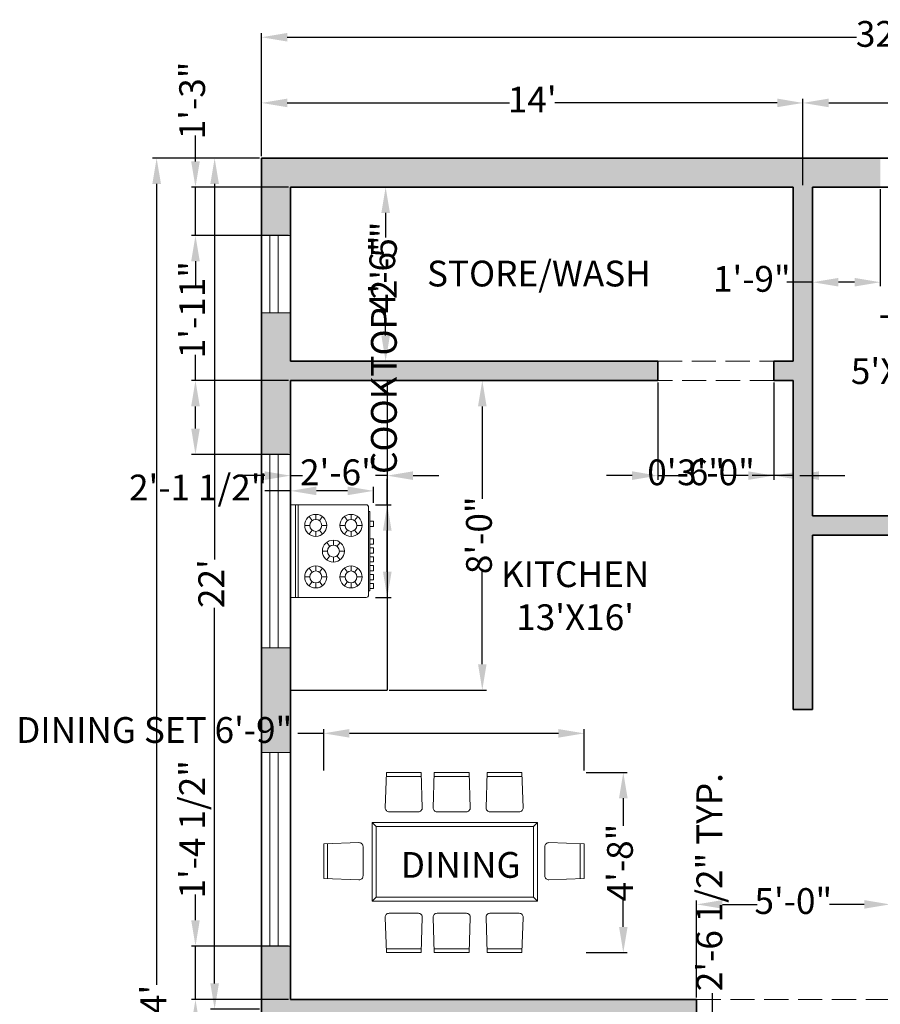
# Model space of a CAD drawing. Units: inches. Extents: x 2073 to 2646, y 2372 to 3017.
# Tile 4 of 8: x 2073 to 2340, y 2686 to 2992. Entities that reach past the tile are written whole.
import ezdxf

# ---------------------------------------------------------------- set-up
doc = ezdxf.new("R2010")
doc.units = ezdxf.units.IN
doc.linetypes.add('DASH', pattern=[0.35, 0.25, -0.1])
for name, color, linetype, lineweight in [('A-ANNO-DIMS', 2, 'Continuous', 18), ('A-AREA-IDEN', 7, 'Continuous', 25), ('A-EQPM', 8, 'Continuous', 18), ('A-FLOR-CASE', 8, 'Continuous', 25), ('A-FURN', 8, 'Continuous', 18), ('A-GLAZ', 4, 'Continuous', 18), ('A-WALL', 7, 'Continuous', 35), ('A-WALL-OVHD', 7, 'DASH', 18), ('A-WALL-PATT', 30, 'Continuous', 13)]:
    doc.layers.add(name, color=color, linetype=linetype, lineweight=lineweight)
doc.styles.get("Standard").update_dxf_attribs({"font": 'arial.ttf'})
doc.dimstyles.new('ISO-25', dxfattribs={"dimtxt": 8, "dimasz": 8, "dimexe": 1.25, "dimexo": 0.625, "dimtad": 0, "dimdec": 1, "dimlunit": 4, "dimtxsty": 'Standard', "dimcen": 2.5, "dimadec": 0, "dimazin": 0, "dimtfac": 1, "dimtdec": 1, "dimtmove": 0, "dimatfit": 3, "dimfxl": 1, "dimarcsym": 0})

# ---------------------------------------------------------------- blocks, each defined once
blk = doc.blocks.new('*D3')
at = {"layer": 'A-ANNO-DIMS', "color": 0, "lineweight": -2, "transparency": 16777216}
for p, q in [((2147.67, 2948.66), (2132.48, 2948.66)), ((2133.73, 2940.66), (2133.73, 2824.15)), ((2133.73, 2692.66), (2133.73, 2809.18)), ((2147.67, 2684.66), (2132.48, 2684.66))]:
    blk.add_line(p, q, dxfattribs=at)
at = {"layer": 'A-ANNO-DIMS', "color": 0, "transparency": 16777216}
for points in [[(2132.4, 2940.66), (2135.06, 2940.66), (2133.73, 2948.66)], [(2132.4, 2692.66), (2135.06, 2692.66), (2133.73, 2684.66)]]:
    blk.add_solid(points, dxfattribs=at)
at = {"layer": 'Defpoints', "color": 0, "transparency": 16777216}
for p in [(2133.73, 2948.66), (2148.29, 2948.66), (2148.29, 2684.66)]:
    blk.add_point(p, dxfattribs=at)
at = {"layer": 'A-ANNO-DIMS', "color": 0, "transparency": 16777216, "insert": (2133.73, 2816.66), "char_height": 8, "attachment_point": 5, "rotation": 90}
blk.add_mtext("22'", dxfattribs=at)
blk = doc.blocks.new('*D4')
at = {"layer": 'A-ANNO-DIMS', "color": 0, "lineweight": -2, "transparency": 16777216}
for p, q in [((2148.29, 2949.29), (2148.29, 2967.03)), ((2156.29, 2965.78), (2225.25, 2965.78)), ((2308.29, 2965.78), (2239.33, 2965.78)), ((2316.29, 2949.29), (2316.29, 2967.03))]:
    blk.add_line(p, q, dxfattribs=at)
at = {"layer": 'A-ANNO-DIMS', "color": 0, "transparency": 16777216}
for points in [[(2156.29, 2967.12), (2156.29, 2964.45), (2148.29, 2965.78)], [(2308.29, 2967.12), (2308.29, 2964.45), (2316.29, 2965.78)]]:
    blk.add_solid(points, dxfattribs=at)
at = {"layer": 'Defpoints', "color": 0, "transparency": 16777216}
for p in [(2316.29, 2965.78), (2148.29, 2948.66), (2316.29, 2948.66)]:
    blk.add_point(p, dxfattribs=at)
at = {"layer": 'A-ANNO-DIMS', "color": 0, "transparency": 16777216, "insert": (2232.29, 2965.78), "char_height": 8, "attachment_point": 5}
blk.add_mtext("14'", dxfattribs=at)
blk = doc.blocks.new('*D5')
at = {"layer": 'A-ANNO-DIMS', "color": 0, "lineweight": -2, "transparency": 16777216}
for p, q in [((2316.29, 2940.29), (2316.29, 2967.03)), ((2324.29, 2965.78), (2347.96, 2965.78)), ((2380.29, 2965.78), (2356.62, 2965.78)), ((2388.29, 2940.29), (2388.29, 2967.03))]:
    blk.add_line(p, q, dxfattribs=at)
at = {"layer": 'A-ANNO-DIMS', "color": 0, "transparency": 16777216}
for points in [[(2324.29, 2967.12), (2324.29, 2964.45), (2316.29, 2965.78)], [(2380.29, 2967.12), (2380.29, 2964.45), (2388.29, 2965.78)]]:
    blk.add_solid(points, dxfattribs=at)
at = {"layer": 'Defpoints', "color": 0, "transparency": 16777216}
for p in [(2388.29, 2965.78), (2316.29, 2939.66), (2388.29, 2939.66)]:
    blk.add_point(p, dxfattribs=at)
at = {"layer": 'A-ANNO-DIMS', "color": 0, "transparency": 16777216, "insert": (2352.29, 2965.78), "char_height": 8, "attachment_point": 5}
blk.add_mtext("6'", dxfattribs=at)
blk = doc.blocks.new('*D7')
at = {"layer": 'A-ANNO-DIMS', "color": 0, "lineweight": -2, "transparency": 16777216}
for p, q in [((2148.29, 2949.29), (2148.29, 2987.4)), ((2532.29, 2950.58), (2532.29, 2987.4)), ((2156.29, 2986.15), (2332.88, 2986.15)), ((2524.29, 2986.15), (2347.7, 2986.15))]:
    blk.add_line(p, q, dxfattribs=at)
at = {"layer": 'A-ANNO-DIMS', "color": 0, "transparency": 16777216}
for points in [[(2156.29, 2987.48), (2156.29, 2984.81), (2148.29, 2986.15)], [(2524.29, 2987.48), (2524.29, 2984.81), (2532.29, 2986.15)]]:
    blk.add_solid(points, dxfattribs=at)
at = {"layer": 'Defpoints', "color": 0, "transparency": 16777216}
for p in [(2148.29, 2986.15), (2148.29, 2948.66), (2532.29, 2949.95)]:
    blk.add_point(p, dxfattribs=at)
at = {"layer": 'A-ANNO-DIMS', "color": 0, "transparency": 16777216, "insert": (2340.29, 2986.15), "char_height": 8, "attachment_point": 5}
blk.add_mtext("32'", dxfattribs=at)
blk = doc.blocks.new('*D8')
at = {"layer": 'A-ANNO-DIMS', "color": 0, "lineweight": -2, "transparency": 16777216}
for p, q in [((2147.67, 2948.66), (2114.49, 2948.66)), ((2115.74, 2940.66), (2115.74, 2692.24)), ((2115.74, 2428.66), (2115.74, 2677.09)), ((2147.67, 2420.66), (2114.49, 2420.66))]:
    blk.add_line(p, q, dxfattribs=at)
at = {"layer": 'A-ANNO-DIMS', "color": 0, "transparency": 16777216}
for points in [[(2114.41, 2940.66), (2117.08, 2940.66), (2115.74, 2948.66)], [(2114.41, 2428.66), (2117.08, 2428.66), (2115.74, 2420.66)]]:
    blk.add_solid(points, dxfattribs=at)
at = {"layer": 'Defpoints', "color": 0, "transparency": 16777216}
for p in [(2148.29, 2948.66), (2115.74, 2420.66), (2148.29, 2420.66)]:
    blk.add_point(p, dxfattribs=at)
at = {"layer": 'A-ANNO-DIMS', "color": 0, "transparency": 16777216, "insert": (2115.74, 2684.66), "char_height": 8, "attachment_point": 5, "rotation": 90}
blk.add_mtext("44'", dxfattribs=at)
blk = doc.blocks.new('g')
at = {"color": 0}
for p, q in [((2245.13, 2782.27), (2273.89, 2782.27)), ((2245.13, 2782.27), (2245.13, 2758.84)), ((2245.13, 2780.69), (2273.89, 2780.69)), ((2245.13, 2779.9), (2273.89, 2779.9)), ((2273.89, 2782.27), (2273.89, 2758.84)), ((2250.05, 2775.56), (2248.8, 2776.51)), ((2251.52, 2777.86), (2251.52, 2776.29)), ((2252.99, 2775.56), (2254.25, 2776.51)), ((2266.03, 2775.56), (2264.77, 2776.51)), ((2267.5, 2777.86), (2267.5, 2776.29)), ((2268.97, 2775.56), (2270.22, 2776.51)), ((2249.68, 2774.44), (2248.1, 2774.44)), ((2254.95, 2774.44), (2253.37, 2774.44)), ((2264.08, 2774.44), (2265.65, 2774.44)), ((2269.35, 2774.44), (2270.92, 2774.44)), ((2248.8, 2772.37), (2250.05, 2773.32)), ((2251.52, 2772.59), (2251.52, 2771.02)), ((2254.25, 2772.37), (2252.99, 2773.32)), ((2258.04, 2770.09), (2256.79, 2771.05)), ((2259.51, 2772.4), (2259.51, 2770.82)), ((2260.98, 2770.09), (2262.24, 2771.05)), ((2264.77, 2772.37), (2266.03, 2773.32)), ((2267.5, 2772.59), (2267.5, 2771.02)), ((2270.22, 2772.37), (2268.97, 2773.32)), ((2257.66, 2768.98), (2256.09, 2768.98)), ((2256.79, 2766.91), (2258.04, 2767.86)), ((2262.24, 2766.91), (2260.98, 2767.86)), ((2262.93, 2768.98), (2261.36, 2768.98)), ((2248.8, 2765.58), (2250.05, 2764.63)), ((2251.52, 2765.36), (2251.52, 2766.94)), ((2254.25, 2765.58), (2252.99, 2764.63)), ((2259.51, 2767.13), (2259.51, 2765.55)), ((2264.77, 2765.58), (2266.03, 2764.63)), ((2267.5, 2765.36), (2267.5, 2766.94)), ((2270.22, 2765.58), (2268.97, 2764.63)), ((2249.68, 2763.51), (2248.1, 2763.51)), ((2250.05, 2762.4), (2248.8, 2761.44)), ((2251.52, 2760.09), (2251.52, 2761.67)), ((2252.99, 2762.4), (2254.25, 2761.44)), ((2254.95, 2763.51), (2253.37, 2763.51)), ((2264.08, 2763.51), (2265.65, 2763.51)), ((2266.03, 2762.4), (2264.77, 2761.44)), ((2267.5, 2760.09), (2267.5, 2761.67)), ((2268.97, 2762.4), (2270.22, 2761.44)), ((2269.35, 2763.51), (2270.92, 2763.51)), ((2245.92, 2758.05), (2273.1, 2758.05)), ((2247.22, 2757.66), (2247.22, 2758.05)), ((2247.22, 2757.66), (2271.8, 2757.66)), ((2247.9, 2757.66), (2247.9, 2756.57)), ((2247.9, 2756.57), (2249.5, 2756.57)), ((2249.5, 2756.57), (2249.5, 2757.66)), ((2250.66, 2757.66), (2250.66, 2756.57)), ((2250.66, 2756.57), (2252.25, 2756.57)), ((2252.25, 2756.57), (2252.25, 2757.66)), ((2253.41, 2757.66), (2253.41, 2756.57)), ((2253.41, 2756.57), (2255.01, 2756.57)), ((2255.01, 2756.57), (2255.01, 2757.66)), ((2256.17, 2757.66), (2256.17, 2756.57)), ((2256.17, 2756.57), (2257.76, 2756.57)), ((2257.76, 2756.57), (2257.76, 2757.66)), ((2258.93, 2757.66), (2258.93, 2756.57)), ((2258.93, 2756.57), (2260.52, 2756.57)), ((2260.52, 2756.57), (2260.52, 2757.66)), ((2261.68, 2757.66), (2261.68, 2756.57)), ((2261.68, 2756.57), (2263.28, 2756.57)), ((2263.28, 2756.57), (2263.28, 2757.66)), ((2267.19, 2757.66), (2267.19, 2756.57)), ((2267.19, 2756.57), (2268.79, 2756.57)), ((2268.79, 2756.57), (2268.79, 2757.66)), ((2271.8, 2757.66), (2271.8, 2758.05))]:
    blk.add_line(p, q, dxfattribs=at)
for centre, radius in [((2251.52, 2774.44), 3.42), ((2267.5, 2774.44), 3.42), ((2251.52, 2774.44), 1.85), ((2267.5, 2774.44), 1.85), ((2259.51, 2768.98), 3.42), ((2259.51, 2768.98), 1.85), ((2251.52, 2763.51), 3.42), ((2251.52, 2763.51), 1.85), ((2267.5, 2763.51), 3.42), ((2267.5, 2763.51), 1.85)]:
    blk.add_circle(centre, radius, dxfattribs=at)
for centre, start, end in [((2245.92, 2758.84), 180, 270), ((2273.1, 2758.84), 270, 0)]:
    blk.add_arc(centre, 0.787, start, end, dxfattribs=at)
blk = doc.blocks.new('8 Person Rec 01')
for p, q in [((-459, 2644), (-509, 2694)), ((441, 2644), (491, 2694)), ((-459, 644), (-509, 594)), ((441, 644), (491, 594))]:
    blk.add_line(p, q)
for points in [[(236, 2863), (221, 3311), (-221, 3311), (-236, 2863, 0.424007), (-186, 2811), (186, 2811, 0.424007)], [(-714, 2529), (-1162, 2514), (-1162, 2073), (-714, 2058, 0.424007), (-662, 2108), (-662, 2479, 0.424007)], [(679, 2529), (1128, 2514), (1128, 2073), (679, 2058, -0.424007), (628, 2108), (628, 2479, -0.424007)], [(-714, 1920), (-1162, 1905), (-1162, 1463), (-714, 1448, 0.424007), (-662, 1498), (-662, 1870, 0.424007)], [(679, 1920), (1128, 1905), (1128, 1463), (679, 1448, -0.424007), (628, 1498), (628, 1870, -0.424007)], [(-714, 1248), (-1162, 1233), (-1162, 791), (-714, 776, 0.424007), (-662, 826), (-662, 1198, 0.424007)], [(679, 1248), (1128, 1233), (1128, 791), (679, 776, -0.424007), (628, 826), (628, 1198, -0.424007)], [(236, 448), (221, 0), (-221, 0), (-236, 448, -0.424007), (-186, 500), (186, 500, -0.424007)]]:
    blk.add_lwpolyline(points, format="xyb", close=True)
for points in [[(-222, 3261), (223, 3261)], [(-1112, 2071), (-1112, 2516)], [(1078, 2071), (1078, 2516)], [(-1112, 1462), (-1112, 1907)], [(1078, 1462), (1078, 1907)], [(-1112, 790), (-1112, 1235)], [(1078, 790), (1078, 1235)], [(-222, 50), (223, 50)]]:
    blk.add_lwpolyline(points)
for points in [[(-509, 594), (491, 594), (491, 2694), (-509, 2694)], [(-459, 644), (441, 644), (441, 2644), (-459, 2644)]]:
    blk.add_lwpolyline(points, close=True)
blk = doc.blocks.new('GLAZ-60IN')
for p, q in [((0, 60), (0, 0)), ((2.6, 60), (2.6, 0))]:
    blk.add_line(p, q)
blk = doc.blocks.new('GLAZ-24IN')
for p, q in [((0, 24), (0, 0)), ((2.6, 24), (2.6, 0))]:
    blk.add_line(p, q)
blk = doc.blocks.new('*D32')
at = {"layer": 'A-ANNO-DIMS', "color": 0, "lineweight": -2, "transparency": 16777216}
for p, q in [((2288.27, 2681.66), (2288.27, 2689.66)), ((2277.03, 2681.66), (2289.52, 2681.66)), ((2288.27, 2659.07), (2288.27, 2673.66)), ((2277.03, 2651.07), (2289.52, 2651.07))]:
    blk.add_line(p, q, dxfattribs=at)
at = {"layer": 'A-ANNO-DIMS', "color": 0, "transparency": 16777216}
for points in [[(2286.93, 2673.66), (2289.6, 2673.66), (2288.27, 2681.66)], [(2286.93, 2659.07), (2289.6, 2659.07), (2288.27, 2651.07)]]:
    blk.add_solid(points, dxfattribs=at)
at = {"layer": 'Defpoints', "color": 0, "transparency": 16777216}
for p in [(2276.41, 2681.66), (2288.27, 2681.66), (2276.41, 2651.07)]:
    blk.add_point(p, dxfattribs=at)
at = {"layer": 'A-ANNO-DIMS', "color": 0, "transparency": 16777216, "insert": (2288.27, 2724.06), "char_height": 8, "attachment_point": 5, "rotation": 90}
blk.add_mtext('2\'-6 1/2" TYP.', dxfattribs=at)
blk = doc.blocks.new('*D37')
at = {"layer": 'A-ANNO-DIMS', "color": 0, "lineweight": -2, "transparency": 16777216}
for p, q in [((2187.3, 2841.12), (2187.3, 2849.12)), ((2183.61, 2841.12), (2188.55, 2841.12)), ((2187.3, 2820.36), (2187.3, 2833.12)), ((2183.61, 2812.36), (2188.55, 2812.36))]:
    blk.add_line(p, q, dxfattribs=at)
at = {"layer": 'A-ANNO-DIMS', "color": 0, "transparency": 16777216}
for points in [[(2185.97, 2833.12), (2188.64, 2833.12), (2187.3, 2841.12)], [(2185.97, 2820.36), (2188.64, 2820.36), (2187.3, 2812.36)]]:
    blk.add_solid(points, dxfattribs=at)
at = {"layer": 'Defpoints', "color": 0, "transparency": 16777216}
for p in [(2182.99, 2841.12), (2187.3, 2841.12), (2182.99, 2812.36)]:
    blk.add_point(p, dxfattribs=at)
at = {"layer": 'A-ANNO-DIMS', "color": 0, "transparency": 16777216, "insert": (2187.3, 2889.83), "char_height": 8, "attachment_point": 5, "rotation": 90}
blk.add_mtext('COOKTOP 2\'-5"', dxfattribs=at)
blk = doc.blocks.new('*D38')
at = {"layer": 'A-ANNO-DIMS', "color": 0, "lineweight": -2, "transparency": 16777216}
for p, q in [((2157.29, 2841.75), (2157.29, 2846.69)), ((2182.99, 2841.75), (2182.99, 2846.69)), ((2157.29, 2845.44), (2149.29, 2845.44)), ((2174.99, 2845.44), (2165.29, 2845.44))]:
    blk.add_line(p, q, dxfattribs=at)
at = {"layer": 'A-ANNO-DIMS', "color": 0, "transparency": 16777216}
for points in [[(2165.29, 2846.77), (2165.29, 2844.1), (2157.29, 2845.44)], [(2174.99, 2846.77), (2174.99, 2844.1), (2182.99, 2845.44)]]:
    blk.add_solid(points, dxfattribs=at)
at = {"layer": 'Defpoints', "color": 0, "transparency": 16777216}
for p in [(2157.29, 2845.44), (2157.29, 2841.12), (2182.99, 2841.12)]:
    blk.add_point(p, dxfattribs=at)
at = {"layer": 'A-ANNO-DIMS', "color": 0, "transparency": 16777216, "insert": (2128.64, 2845.44), "char_height": 8, "attachment_point": 5}
blk.add_mtext('2\'-1 1/2"', dxfattribs=at)
blk = doc.blocks.new('*D39')
at = {"layer": 'A-ANNO-DIMS', "color": 0, "lineweight": -2, "transparency": 16777216}
for p, q in [((2167.57, 2758.72), (2167.57, 2771.47)), ((2248.41, 2758.72), (2248.41, 2771.47)), ((2167.57, 2770.22), (2159.57, 2770.22)), ((2240.41, 2770.22), (2175.57, 2770.22))]:
    blk.add_line(p, q, dxfattribs=at)
at = {"layer": 'A-ANNO-DIMS', "color": 0, "transparency": 16777216}
for points in [[(2175.57, 2771.55), (2175.57, 2768.89), (2167.57, 2770.22)], [(2240.41, 2771.55), (2240.41, 2768.89), (2248.41, 2770.22)]]:
    blk.add_solid(points, dxfattribs=at)
at = {"layer": 'Defpoints', "color": 0, "transparency": 16777216}
for p in [(2167.57, 2770.22), (2167.57, 2758.09), (2248.41, 2758.09)]:
    blk.add_point(p, dxfattribs=at)
at = {"layer": 'A-ANNO-DIMS', "color": 0, "transparency": 16777216, "insert": (2114.98, 2770.22), "char_height": 8, "attachment_point": 5}
blk.add_mtext('DINING SET 6\'-9"', dxfattribs=at)
blk = doc.blocks.new('*D40')
at = {"layer": 'A-ANNO-DIMS', "color": 0, "lineweight": -2, "transparency": 16777216}
for p, q in [((2249.04, 2758.09), (2261.79, 2758.09)), ((2260.54, 2750.09), (2260.54, 2741.56)), ((2260.54, 2710.19), (2260.54, 2718.72)), ((2249.04, 2702.19), (2261.79, 2702.19))]:
    blk.add_line(p, q, dxfattribs=at)
at = {"layer": 'A-ANNO-DIMS', "color": 0, "transparency": 16777216}
for points in [[(2259.21, 2750.09), (2261.87, 2750.09), (2260.54, 2758.09)], [(2259.21, 2710.19), (2261.87, 2710.19), (2260.54, 2702.19)]]:
    blk.add_solid(points, dxfattribs=at)
at = {"layer": 'Defpoints', "color": 0, "transparency": 16777216}
for p in [(2248.41, 2758.09), (2260.54, 2758.09), (2248.41, 2702.19)]:
    blk.add_point(p, dxfattribs=at)
at = {"layer": 'A-ANNO-DIMS', "color": 0, "transparency": 16777216, "insert": (2260.54, 2730.14), "char_height": 8, "attachment_point": 5, "rotation": 90}
blk.add_mtext('4\'-8"', dxfattribs=at)
blk = doc.blocks.new('*D44')
at = {"layer": 'A-ANNO-DIMS', "color": 0, "lineweight": -2, "transparency": 16777216}
for p, q in [((2157.92, 2939.66), (2188.04, 2939.66)), ((2186.79, 2931.66), (2186.79, 2924.08)), ((2186.79, 2893.66), (2186.79, 2901.25)), ((2157.92, 2885.66), (2188.04, 2885.66))]:
    blk.add_line(p, q, dxfattribs=at)
at = {"layer": 'A-ANNO-DIMS', "color": 0, "transparency": 16777216}
for points in [[(2185.46, 2931.66), (2188.12, 2931.66), (2186.79, 2939.66)], [(2185.46, 2893.66), (2188.12, 2893.66), (2186.79, 2885.66)]]:
    blk.add_solid(points, dxfattribs=at)
at = {"layer": 'Defpoints', "color": 0, "transparency": 16777216}
for p in [(2157.29, 2939.66), (2157.29, 2885.66), (2186.79, 2885.66)]:
    blk.add_point(p, dxfattribs=at)
at = {"layer": 'A-ANNO-DIMS', "color": 0, "transparency": 16777216, "insert": (2186.79, 2912.66), "char_height": 8, "attachment_point": 5, "rotation": 90}
blk.add_mtext('4\'-6"', dxfattribs=at)
blk = doc.blocks.new('*D52')
at = {"layer": 'A-ANNO-DIMS', "color": 0, "lineweight": -2, "transparency": 16777216}
for p, q in [((2283.29, 2688.29), (2283.29, 2718.41)), ((2343.29, 2688.29), (2343.29, 2718.41)), ((2291.29, 2717.16), (2302.03, 2717.16)), ((2335.29, 2717.16), (2324.55, 2717.16))]:
    blk.add_line(p, q, dxfattribs=at)
at = {"layer": 'A-ANNO-DIMS', "color": 0, "transparency": 16777216}
for points in [[(2291.29, 2718.5), (2291.29, 2715.83), (2283.29, 2717.16)], [(2335.29, 2718.5), (2335.29, 2715.83), (2343.29, 2717.16)]]:
    blk.add_solid(points, dxfattribs=at)
at = {"layer": 'Defpoints', "color": 0, "transparency": 16777216}
for p in [(2343.29, 2717.16), (2283.29, 2687.66), (2343.29, 2687.66)]:
    blk.add_point(p, dxfattribs=at)
at = {"layer": 'A-ANNO-DIMS', "color": 0, "transparency": 16777216, "insert": (2313.29, 2717.16), "char_height": 8, "attachment_point": 5}
blk.add_mtext('5\'-0"', dxfattribs=at)
blk = doc.blocks.new('*D60')
at = {"layer": 'A-ANNO-DIMS', "color": 0, "lineweight": -2, "transparency": 16777216}
for p, q in [((2127.79, 2712.25), (2127.79, 2720.25)), ((2156.67, 2704.25), (2126.54, 2704.25)), ((2127.79, 2687.66), (2127.79, 2704.25)), ((2156.67, 2687.66), (2126.54, 2687.66)), ((2127.79, 2679.66), (2127.79, 2671.66))]:
    blk.add_line(p, q, dxfattribs=at)
at = {"layer": 'A-ANNO-DIMS', "color": 0, "transparency": 16777216}
for points in [[(2126.46, 2712.25), (2129.12, 2712.25), (2127.79, 2704.25)], [(2126.46, 2679.66), (2129.12, 2679.66), (2127.79, 2687.66)]]:
    blk.add_solid(points, dxfattribs=at)
at = {"layer": 'Defpoints', "color": 0, "transparency": 16777216}
for p in [(2127.79, 2704.25), (2157.29, 2704.25), (2157.29, 2687.66)]:
    blk.add_point(p, dxfattribs=at)
at = {"layer": 'A-ANNO-DIMS', "color": 0, "transparency": 16777216, "insert": (2127.79, 2740.45), "char_height": 8, "attachment_point": 5, "rotation": 90}
blk.add_mtext('1\'-4 1/2"', dxfattribs=at)
blk = doc.blocks.new('*D61')
at = {"layer": 'A-ANNO-DIMS', "color": 0, "lineweight": -2, "transparency": 16777216}
for p, q in [((2127.79, 2879.66), (2127.79, 2887.66)), ((2156.67, 2879.66), (2126.54, 2879.66)), ((2127.79, 2864.74), (2127.79, 2871.66)), ((2156.67, 2856.74), (2126.54, 2856.74))]:
    blk.add_line(p, q, dxfattribs=at)
at = {"layer": 'A-ANNO-DIMS', "color": 0, "transparency": 16777216}
for points in [[(2126.46, 2871.66), (2129.12, 2871.66), (2127.79, 2879.66)], [(2126.46, 2864.74), (2129.12, 2864.74), (2127.79, 2856.74)]]:
    blk.add_solid(points, dxfattribs=at)
at = {"layer": 'Defpoints', "color": 0, "transparency": 16777216}
for p in [(2127.79, 2879.66), (2157.29, 2879.66), (2157.29, 2856.74)]:
    blk.add_point(p, dxfattribs=at)
at = {"layer": 'A-ANNO-DIMS', "color": 0, "transparency": 16777216, "insert": (2127.79, 2901.65), "char_height": 8, "attachment_point": 5, "rotation": 90}
blk.add_mtext('1\'-11"', dxfattribs=at)
blk = doc.blocks.new('*D62')
at = {"layer": 'A-ANNO-DIMS', "color": 0, "lineweight": -2, "transparency": 16777216}
for p, q in [((2127.79, 2947.66), (2127.79, 2955.66)), ((2156.67, 2939.66), (2126.54, 2939.66)), ((2127.79, 2924.66), (2127.79, 2939.66)), ((2156.67, 2924.66), (2126.54, 2924.66)), ((2127.79, 2916.66), (2127.79, 2908.66))]:
    blk.add_line(p, q, dxfattribs=at)
at = {"layer": 'A-ANNO-DIMS', "color": 0, "transparency": 16777216}
for points in [[(2126.46, 2947.66), (2129.12, 2947.66), (2127.79, 2939.66)], [(2126.46, 2916.66), (2129.12, 2916.66), (2127.79, 2924.66)]]:
    blk.add_solid(points, dxfattribs=at)
at = {"layer": 'Defpoints', "color": 0, "transparency": 16777216}
for p in [(2127.79, 2939.66), (2157.29, 2939.66), (2157.29, 2924.66)]:
    blk.add_point(p, dxfattribs=at)
at = {"layer": 'A-ANNO-DIMS', "color": 0, "transparency": 16777216, "insert": (2127.79, 2966.55), "char_height": 8, "attachment_point": 5, "rotation": 90}
blk.add_mtext('1\'-3"', dxfattribs=at)
blk = doc.blocks.new('*D63')
at = {"layer": 'A-ANNO-DIMS', "color": 0, "lineweight": -2, "transparency": 16777216}
for p, q in [((2319.29, 2939.04), (2319.29, 2908.91)), ((2340.29, 2939.04), (2340.29, 2908.91)), ((2319.29, 2910.16), (2311.29, 2910.16)), ((2332.29, 2910.16), (2327.29, 2910.16))]:
    blk.add_line(p, q, dxfattribs=at)
at = {"layer": 'A-ANNO-DIMS', "color": 0, "transparency": 16777216}
for points in [[(2327.29, 2911.5), (2327.29, 2908.83), (2319.29, 2910.16)], [(2332.29, 2911.5), (2332.29, 2908.83), (2340.29, 2910.16)]]:
    blk.add_solid(points, dxfattribs=at)
at = {"layer": 'Defpoints', "color": 0, "transparency": 16777216}
for p in [(2319.29, 2939.66), (2340.29, 2939.66), (2319.29, 2910.16)]:
    blk.add_point(p, dxfattribs=at)
at = {"layer": 'A-ANNO-DIMS', "color": 0, "transparency": 16777216, "insert": (2300.41, 2910.16), "char_height": 8, "attachment_point": 5}
blk.add_mtext('1\'-9"', dxfattribs=at)
blk = doc.blocks.new('*D64')
at = {"layer": 'A-ANNO-DIMS', "color": 0, "lineweight": -2, "transparency": 16777216}
for p, q in [((2271.29, 2879.04), (2271.29, 2848.91)), ((2307.29, 2879.04), (2307.29, 2848.91)), ((2263.29, 2850.16), (2255.29, 2850.16)), ((2271.29, 2850.16), (2278.03, 2850.16)), ((2307.29, 2850.16), (2300.55, 2850.16)), ((2315.29, 2850.16), (2323.29, 2850.16))]:
    blk.add_line(p, q, dxfattribs=at)
at = {"layer": 'A-ANNO-DIMS', "color": 0, "transparency": 16777216}
for points in [[(2263.29, 2851.5), (2263.29, 2848.83), (2271.29, 2850.16)], [(2315.29, 2851.5), (2315.29, 2848.83), (2307.29, 2850.16)]]:
    blk.add_solid(points, dxfattribs=at)
at = {"layer": 'Defpoints', "color": 0, "transparency": 16777216}
for p in [(2271.29, 2879.66), (2307.29, 2879.66), (2271.29, 2850.16)]:
    blk.add_point(p, dxfattribs=at)
at = {"layer": 'A-ANNO-DIMS', "color": 0, "transparency": 16777216, "insert": (2289.29, 2850.16), "char_height": 8, "attachment_point": 5}
blk.add_mtext('3\'-0"', dxfattribs=at)
blk = doc.blocks.new('*D65')
at = {"layer": 'A-ANNO-DIMS', "color": 0, "lineweight": -2, "transparency": 16777216}
for p, q in [((2187.92, 2879.66), (2218.04, 2879.66)), ((2216.79, 2871.66), (2216.79, 2842.93)), ((2216.79, 2791.66), (2216.79, 2820.4)), ((2187.92, 2783.66), (2218.04, 2783.66))]:
    blk.add_line(p, q, dxfattribs=at)
at = {"layer": 'A-ANNO-DIMS', "color": 0, "transparency": 16777216}
for points in [[(2215.46, 2871.66), (2218.12, 2871.66), (2216.79, 2879.66)], [(2215.46, 2791.66), (2218.12, 2791.66), (2216.79, 2783.66)]]:
    blk.add_solid(points, dxfattribs=at)
at = {"layer": 'Defpoints', "color": 0, "transparency": 16777216}
for p in [(2187.29, 2879.66), (2187.29, 2783.66), (2216.79, 2783.66)]:
    blk.add_point(p, dxfattribs=at)
at = {"layer": 'A-ANNO-DIMS', "color": 0, "transparency": 16777216, "insert": (2216.79, 2831.66), "char_height": 8, "attachment_point": 5, "rotation": 90}
blk.add_mtext('8\'-0"', dxfattribs=at)
blk = doc.blocks.new('*D66')
at = {"layer": 'A-ANNO-DIMS', "color": 0, "lineweight": -2, "transparency": 16777216}
for p, q in [((2157.29, 2879.04), (2157.29, 2848.91)), ((2187.29, 2879.04), (2187.29, 2848.91)), ((2149.29, 2850.16), (2141.29, 2850.16)), ((2157.29, 2850.16), (2160.96, 2850.16)), ((2187.29, 2850.16), (2183.62, 2850.16)), ((2195.29, 2850.16), (2203.29, 2850.16))]:
    blk.add_line(p, q, dxfattribs=at)
at = {"layer": 'A-ANNO-DIMS', "color": 0, "transparency": 16777216}
for points in [[(2149.29, 2851.5), (2149.29, 2848.83), (2157.29, 2850.16)], [(2195.29, 2851.5), (2195.29, 2848.83), (2187.29, 2850.16)]]:
    blk.add_solid(points, dxfattribs=at)
at = {"layer": 'Defpoints', "color": 0, "transparency": 16777216}
for p in [(2157.29, 2879.66), (2187.29, 2879.66), (2157.29, 2850.16)]:
    blk.add_point(p, dxfattribs=at)
at = {"layer": 'A-ANNO-DIMS', "color": 0, "transparency": 16777216, "insert": (2172.29, 2850.16), "char_height": 8, "attachment_point": 5}
blk.add_mtext('2\'-6"', dxfattribs=at)
blk = doc.blocks.new('*D69')
at = {"layer": 'A-ANNO-DIMS', "color": 0, "lineweight": -2, "transparency": 16777216}
for p, q in [((2307.29, 2879.04), (2307.29, 2848.91)), ((2313.29, 2879.04), (2313.29, 2848.91)), ((2299.29, 2850.16), (2291.29, 2850.16)), ((2313.29, 2850.16), (2307.29, 2850.16)), ((2321.29, 2850.16), (2329.29, 2850.16))]:
    blk.add_line(p, q, dxfattribs=at)
at = {"layer": 'A-ANNO-DIMS', "color": 0, "transparency": 16777216}
for points in [[(2299.29, 2851.5), (2299.29, 2848.83), (2307.29, 2850.16)], [(2321.29, 2851.5), (2321.29, 2848.83), (2313.29, 2850.16)]]:
    blk.add_solid(points, dxfattribs=at)
at = {"layer": 'Defpoints', "color": 0, "transparency": 16777216}
for p in [(2307.29, 2879.66), (2313.29, 2879.66), (2307.29, 2850.16)]:
    blk.add_point(p, dxfattribs=at)
at = {"layer": 'A-ANNO-DIMS', "color": 0, "transparency": 16777216, "insert": (2280.03, 2850.16), "char_height": 8, "attachment_point": 5}
blk.add_mtext('0\'-6"', dxfattribs=at)

msp = doc.modelspace()

# ---------------------------------------------------------------- hatches: boundary and pattern name
at = {"layer": 'A-WALL-PATT'}
h = msp.add_hatch(color=256, dxfattribs=at)
h.dxf.hatch_style = 1
h.paths.add_polyline_path([(2340.29, 2948.66), (2148.29, 2948.66), (2148.29, 2924.66), (2157.29, 2924.66), (2157.29, 2939.66), (2313.29, 2939.66), (2313.29, 2885.66), (2307.29, 2885.66), (2307.29, 2879.66), (2313.29, 2879.66), (2313.29, 2777.66), (2319.29, 2777.66), (2319.29, 2831.66), (2385.29, 2831.66), (2385.29, 2825.68), (2390.69, 2825.68, -0.004149), (2391.29, 2825.68), (2391.29, 2843.66), (2385.29, 2843.66), (2385.29, 2837.66), (2319.29, 2837.66), (2319.29, 2939.66), (2340.29, 2939.66)])
h.paths.add_polyline_path([(2271.29, 2885.66), (2157.29, 2885.66), (2157.29, 2900.66), (2148.29, 2900.66), (2148.29, 2856.74), (2157.29, 2856.74), (2157.29, 2879.66), (2271.29, 2879.66)], flags=17)
h.paths.add_polyline_path([(2157.29, 2796.74), (2148.29, 2796.74), (2148.29, 2764.25), (2157.29, 2764.25)])
h.paths.add_polyline_path([(2157.29, 2681.66), (2283.29, 2681.66), (2283.29, 2687.66), (2157.29, 2687.66), (2157.29, 2704.25), (2148.29, 2704.25), (2148.29, 2621.66), (2157.29, 2621.66)])
h.paths.add_polyline_path([(2196.29, 2501.66), (2157.29, 2501.66), (2157.29, 2561.66), (2148.29, 2561.66), (2148.29, 2492.66), (2196.29, 2492.66)])
h.paths.add_polyline_path([(2295.23, 2495.54), (2295.23, 2501.66), (2256.29, 2501.66), (2256.29, 2492.66), (2295.23, 2492.66)])
h.paths.add_polyline_path([(2355.29, 2603.66), (2361.29, 2603.66), (2361.29, 2609.66), (2355.29, 2609.66), (2355.29, 2639.66), (2349.29, 2639.66), (2349.29, 2501.66), (2343.29, 2501.66), (2343.29, 2492.66), (2349.29, 2492.66), (2349.29, 2420.66), (2532.29, 2420.66), (2532.29, 2486.66), (2523.29, 2486.66), (2523.29, 2429.66), (2355.29, 2429.66)])
h.paths.add_polyline_path([(2532.29, 2633.66), (2523.29, 2633.66), (2523.29, 2609.66), (2439.29, 2609.66), (2439.29, 2615.66), (2433.29, 2615.66), (2433.29, 2609.66), (2397.31, 2609.66), (2397.31, 2604.26, -0.004149), (2397.3, 2603.66), (2523.29, 2603.66), (2523.29, 2546.66), (2532.29, 2546.66)], flags=17)
h.paths.add_polyline_path([(2532.29, 2702.66), (2523.29, 2702.66), (2523.29, 2687.66), (2385.29, 2687.66), (2343.29, 2687.66), (2343.29, 2681.66), (2349.29, 2681.66), (2349.29, 2675.66), (2355.29, 2675.66), (2355.29, 2681.66), (2433.29, 2681.66), (2433.29, 2645.66), (2439.29, 2645.66), (2439.29, 2681.66), (2523.29, 2681.66), (2523.29, 2657.66), (2532.29, 2657.66)])
h.paths.add_polyline_path([(2532.29, 2831.66), (2523.29, 2831.66), (2523.29, 2783.66), (2391.29, 2783.66), (2391.29, 2789.66), (2385.29, 2789.66), (2385.29, 2777.66), (2523.29, 2777.66), (2523.29, 2762.66), (2532.29, 2762.66)])
h.paths.add_polyline_path([(2532.29, 2948.66), (2364.29, 2948.66), (2364.29, 2939.66), (2385.29, 2939.66), (2385.29, 2873.66), (2391.29, 2873.66), (2391.29, 2939.66), (2523.29, 2939.66), (2523.29, 2891.66), (2532.29, 2891.66)])

# ---------------------------------------------------------------- linework, layer by layer
at = {"layer": 'A-FLOR-CASE'}
for p in [(2187.29, 2879.66), (2157.29, 2783.66)]:
    msp.add_line(p, (2187.29, 2783.66), dxfattribs=at)
at = {"layer": 'A-GLAZ'}
for p, q in [((2157.29, 2924.66), (2148.29, 2924.66)), ((2157.29, 2900.66), (2148.29, 2900.66)), ((2157.29, 2856.74), (2148.29, 2856.74)), ((2157.29, 2796.74), (2148.29, 2796.74)), ((2157.29, 2764.25), (2148.29, 2764.25)), ((2157.29, 2704.25), (2148.29, 2704.25))]:
    msp.add_line(p, q, dxfattribs=at)
at = {"layer": 'A-WALL'}
for p, q in [((2532.29, 2948.66), (2148.29, 2948.66)), ((2148.29, 2948.66), (2148.29, 2420.66)), ((2157.29, 2939.66), (2157.29, 2885.66)), ((2313.29, 2939.66), (2157.29, 2939.66)), ((2313.29, 2939.66), (2313.29, 2885.66)), ((2319.29, 2939.66), (2319.29, 2837.66)), ((2385.29, 2939.66), (2319.29, 2939.66)), ((2157.29, 2885.66), (2271.29, 2885.66)), ((2271.29, 2885.66), (2271.29, 2879.66)), ((2307.29, 2885.66), (2307.29, 2879.66)), ((2307.29, 2885.66), (2313.29, 2885.66)), ((2157.29, 2879.66), (2271.29, 2879.66)), ((2157.29, 2879.66), (2157.29, 2687.66)), ((2307.29, 2879.66), (2313.29, 2879.66)), ((2313.29, 2879.66), (2313.29, 2777.66)), ((2385.29, 2837.66), (2319.29, 2837.66)), ((2385.29, 2831.66), (2319.29, 2831.66)), ((2319.29, 2831.66), (2319.29, 2777.66)), ((2319.29, 2777.66), (2313.29, 2777.66)), ((2157.29, 2687.66), (2283.29, 2687.66)), ((2283.29, 2687.66), (2283.29, 2681.66))]:
    msp.add_line(p, q, dxfattribs=at)
at = {"layer": 'A-WALL-OVHD', "ltscale": 30}
for points in [[(2271.29, 2885.66), (2307.29, 2885.66), (2307.29, 2879.66), (2271.29, 2879.66)], [(2283.29, 2687.66), (2343.29, 2687.66), (2343.29, 2681.66), (2283.29, 2681.66)]]:
    msp.add_lwpolyline(points, close=True, dxfattribs=at)

# ---------------------------------------------------------------- block references
at = {"layer": 'A-EQPM', "rotation": 90}
msp.add_blockref('g', (4939.56, 567.23), dxfattribs=at)
at = {"layer": 'A-FURN', "xscale": 0.0244145970643334, "yscale": 0.0244145970643334, "zscale": 0.0244145970643334, "rotation": 90}
msp.add_blockref('8 Person Rec 01', (2248.41, 2730.56), dxfattribs=at)
at = {"layer": 'A-GLAZ'}
for name, p in [('GLAZ-24IN', (2150.89, 2900.66)), ('GLAZ-60IN', (2150.89, 2796.74)), ('GLAZ-60IN', (2150.89, 2704.25))]:
    msp.add_blockref(name, p, dxfattribs=at)

# ---------------------------------------------------------------- texts
at = {"layer": 'A-AREA-IDEN', "char_height": 8, "attachment_point": 1}
for s, insert in [('\\pxqc;STORE/WASH', (2197.27, 2916.85)), ('\\pxqc;T/B\\P5\'X8\'6"', (2311.89, 2899.91)), ("\\pxqc;KITCHEN\\P13'X16'", (2208.5, 2823.58)), ('\\pxqc;DINING', (2173.01, 2733.4))]:
    msp.add_mtext_dynamic_manual_height_columns(s, width=74.1792, gutter_width=12.5, heights=[0], dxfattribs=dict(at, insert=insert))

# ---------------------------------------------------------------- dimensions: what is measured, and where the dimension line sits
at = {"layer": 'A-ANNO-DIMS'}
for base, p1, p2, override, picture, middle in [((2148.29, 2986.15), (2532.29, 2949.95), (2148.29, 2948.66), {"dimclrd": 0, "dimclre": 0, "dimclrt": 0}, '*D7', (2340.29, 2986.15)), ((2316.29, 2965.78), (2148.29, 2948.66), (2316.29, 2948.66), {"dimclrd": 0, "dimclre": 0, "dimclrt": 0}, '*D4', (2232.29, 2965.78)), ((2388.29, 2965.78), (2316.29, 2939.66), (2388.29, 2939.66), {"dimclrd": 0, "dimclre": 0, "dimclrt": 0}, '*D5', (2352.29, 2965.78)), ((2343.29, 2717.16), (2283.29, 2687.66), (2343.29, 2687.66), {"dimdec": 1, "dimlfac": 1, "dimrnd": 0, "dimzin": 1, "dimdsep": 46, "dimlunit": 4, "dimfrac": 2}, '*D52', (2313.29, 2717.16))]:
    dim = msp.add_linear_dim(base=base, p1=p1, p2=p2, dimstyle='ISO-25', override=override, dxfattribs=at)
    dim.commit()
    dim.dimension.update_dxf_attribs({"geometry": picture, "text_midpoint": middle})
for base, p1, p2, angle, override, picture, middle in [((2127.79, 2939.66), (2157.29, 2924.66), (2157.29, 2939.66), 90, {"dimdec": 1, "dimlfac": 1, "dimrnd": 0, "dimzin": 1, "dimdsep": 46, "dimlunit": 4, "dimfrac": 2}, '*D62', (2127.79, 2966.55)), ((2115.74, 2420.66), (2148.29, 2948.66), (2148.29, 2420.66), 90, {"dimclrd": 0, "dimclre": 0, "dimclrt": 0}, '*D8', (2115.74, 2684.66)), ((2133.73, 2948.66), (2148.29, 2684.66), (2148.29, 2948.66), 90, {"dimclrd": 0, "dimclre": 0, "dimclrt": 0}, '*D3', (2133.73, 2816.66)), ((2186.79, 2885.66), (2157.29, 2939.66), (2157.29, 2885.66), 270, {"dimdec": 1, "dimlfac": 1, "dimrnd": 0, "dimzin": 1, "dimdsep": 46, "dimlunit": 4, "dimfrac": 2}, '*D44', (2186.79, 2912.66)), ((2319.29, 2910.16), (2340.29, 2939.66), (2319.29, 2939.66), 180, {"dimdec": 1, "dimlfac": 1, "dimrnd": 0, "dimzin": 1, "dimdsep": 46, "dimlunit": 4, "dimfrac": 2}, '*D63', (2300.41, 2910.16)), ((2127.79, 2879.66), (2157.29, 2856.74), (2157.29, 2879.66), 90, {"dimdec": 1, "dimlfac": 1, "dimrnd": 0, "dimzin": 1, "dimdsep": 46, "dimlunit": 4, "dimfrac": 2}, '*D61', (2127.79, 2901.65)), ((2157.29, 2850.16), (2187.29, 2879.66), (2157.29, 2879.66), 180, {"dimdec": 1, "dimlfac": 1, "dimrnd": 0, "dimzin": 1, "dimdsep": 46, "dimlunit": 4, "dimfrac": 2}, '*D66', (2172.29, 2850.16)), ((2216.79, 2783.66), (2187.29, 2879.66), (2187.29, 2783.66), 270, {"dimdec": 1, "dimlfac": 1, "dimrnd": 0, "dimzin": 1, "dimdsep": 46, "dimlunit": 4, "dimfrac": 2}, '*D65', (2216.79, 2831.66)), ((2271.29, 2850.16), (2307.29, 2879.66), (2271.29, 2879.66), 180, {"dimdec": 1, "dimlfac": 1, "dimrnd": 0, "dimzin": 1, "dimdsep": 46, "dimlunit": 4, "dimfrac": 2}, '*D64', (2289.29, 2850.16)), ((2307.29, 2850.16), (2313.29, 2879.66), (2307.29, 2879.66), 180, {"dimdec": 1, "dimlfac": 1, "dimrnd": 0, "dimzin": 1, "dimdsep": 46, "dimlunit": 4, "dimfrac": 2}, '*D69', (2280.03, 2850.16)), ((2157.29, 2845.44), (2182.99, 2841.12), (2157.29, 2841.12), 180, {"dimdec": 1, "dimlfac": 1, "dimrnd": 0, "dimzin": 1, "dimdsep": 46, "dimlunit": 4, "dimfrac": 2}, '*D38', (2128.64, 2845.44)), ((2127.79, 2704.25), (2157.29, 2687.66), (2157.29, 2704.25), 90, {"dimdec": 1, "dimlfac": 1, "dimrnd": 0, "dimzin": 1, "dimdsep": 46, "dimlunit": 4, "dimfrac": 2}, '*D60', (2127.79, 2740.45)), ((2260.54, 2758.09), (2248.41, 2702.19), (2248.41, 2758.09), 90, {"dimdec": 1, "dimlfac": 1, "dimrnd": 0, "dimzin": 1, "dimdsep": 46, "dimlunit": 4, "dimfrac": 2}, '*D40', (2260.54, 2730.14))]:
    dim = msp.add_linear_dim(base=base, p1=p1, p2=p2, angle=angle, dimstyle='ISO-25', override=override, dxfattribs=at)
    dim.commit()
    dim.dimension.update_dxf_attribs({"geometry": picture, "text_midpoint": middle})
for base, p1, p2, angle, text, picture, middle in [((2187.3, 2841.12), (2182.99, 2812.36), (2182.99, 2841.12), 90, 'COOKTOP <>', '*D37', (2187.3, 2889.83)), ((2167.57, 2770.22), (2248.41, 2758.09), (2167.57, 2758.09), 180, 'DINING SET <>', '*D39', (2114.98, 2770.22)), ((2288.27, 2681.66), (2276.41, 2651.07), (2276.41, 2681.66), 90, '<> TYP.', '*D32', (2288.27, 2724.06))]:
    dim = msp.add_linear_dim(base=base, p1=p1, p2=p2, angle=angle, text=text, dimstyle='ISO-25', override={"dimdec": 1, "dimlfac": 1, "dimrnd": 0, "dimzin": 1, "dimdsep": 46, "dimlunit": 4, "dimfrac": 2}, dxfattribs=at)
    dim.commit()
    dim.dimension.update_dxf_attribs({"geometry": picture, "text_midpoint": middle})

doc.saveas('drawing.dxf')
